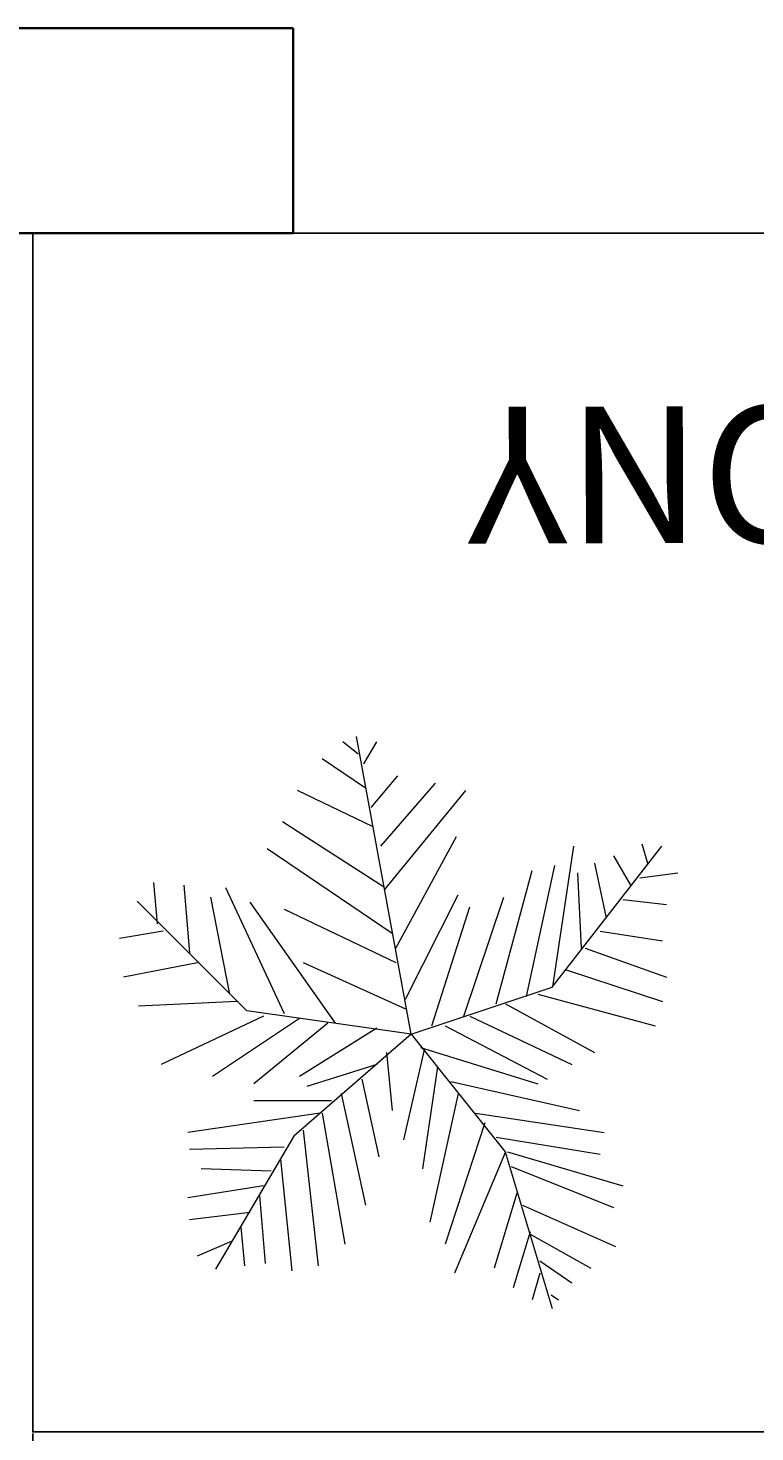
# Model space of a CAD drawing. Units: inches. Extents: x 4159 to 4826, y 299 to 1026.
# Tile 3 of 37: x 4268 to 4300, y 340 to 401. Entities that reach past the tile are written whole.
import ezdxf

# ---------------------------------------------------------------- set-up
doc = ezdxf.new("R2010")
doc.units = ezdxf.units.IN
for name, color, linetype, lineweight in [('A-ANNO-DIMS', 2, 'Continuous', 18), ('A-AREA-IDEN', 7, 'Continuous', 18), ('A-FLOR-BALC', 7, 'Continuous', 25), ('A-WALL', 7, 'Continuous', 35), ('L-PLNT', 94, 'Continuous', 13)]:
    doc.layers.add(name, color=color, linetype=linetype, lineweight=lineweight)
doc.styles.get("Standard").update_dxf_attribs({"font": 'arial.ttf'})
doc.dimstyles.get("Standard").update_dxf_attribs({"dimtxt": 0.18, "dimasz": 0.18, "dimexe": 0.18, "dimexo": 0.0625, "dimgap": 0.09, "dimtad": 0, "dimtih": 1, "dimtoh": 1, "dimdec": 4, "dimzin": 0, "dimdsep": 46, "dimtxsty": 'Standard', "dimcen": 0.09, "dimadec": 0, "dimazin": 0, "dimtfac": 1, "dimtdec": 4, "dimtofl": 0, "dimtmove": 0, "dimatfit": 3, "dimfxl": 1, "dimtolj": 1, "dimtzin": 0, "dimarcsym": 0})

# ---------------------------------------------------------------- blocks, each defined once
blk = doc.blocks.new('*U12')
for p, q in [((0, 0), (-10.5, 57)), ((-10.186, 53.64), (-13.084, 55.962)), ((-9.099, 51.782), (-6.563, 55.962)), ((-8.737, 47.138), (-17.069, 52.711)), ((-7.65, 43.423), (-2.578, 49.46)), ((-7.288, 39.707), (-21.778, 46.673)), ((-5.839, 35.992), (4.667, 48.067)), ((-5.114, 27.632), (10.463, 46.673)), ((-5.114, 28.097), (-24.676, 40.636)), ((-2.941, 16.486), (8.652, 37.85)), ((-3.665, 19.273), (-27.574, 35.527)), ((27, 9), (48, 36)), ((27.127, 9.056), (31.112, 35.992)), ((44.153, 36.456), (45.239, 32.741)), ((22.055, 7.198), (27.489, 32.277)), ((35.096, 32.741), (37.27, 22.524)), ((38.719, 34.134), (41.979, 28.561)), ((16.259, 5.805), (23.142, 31.348)), ((31.836, 30.883), (32.561, 16.486)), ((43.791, 29.954), (51.036, 30.883)), ((-48.585, 21.131), (-49.309, 29.026)), ((-43.513, 28.561), (-42.427, 15.558)), ((-35.544, 28.097), (-24.314, 3.947)), ((-31.5, 4.5), (-52.5, 25.5)), ((-38.442, 26.239), (-34.819, 7.663)), ((-14.533, 2.09), (-30.834, 25.31)), ((-1.129, 6.734), (9.014, 26.704)), ((3.942, 1.625), (11.187, 24.381)), ((10.101, 3.483), (17.708, 26.239)), ((40.53, 25.775), (48.862, 24.846)), ((-24.314, 23.917), (-2.941, 13.7)), ((-47.498, 19.737), (-55.83, 18.344)), ((36.183, 19.737), (48.137, 17.88)), ((33.285, 16.486), (48.862, 10.913)), ((-40.615, 13.7), (-55.105, 10.913)), ((-20.691, 13.7), (-1.129, 4.876)), ((29.662, 12.307), (48.137, 6.269)), ((0, 0), (27, 9)), ((-33.37, 6.269), (-52.207, 5.34)), ((18.07, 5.805), (35.096, -3.483)), ((24.229, 7.663), (46.688, 1.625)), ((-28.299, 3.483), (-47.86, -5.805)), ((-21.416, 3.018), (-38.079, -8.128)), ((0, 0), (-31.5, 4.5)), ((11.187, 3.483), (30.749, -5.805)), ((-15.982, 2.09), (-30.11, -9.521)), ((0, 0), (-22.5, -19.5)), ((-6.563, 1.161), (-21.416, -8.128)), ((0, 0), (18, -22.5)), ((6.478, 1.625), (26.04, -8.592)), ((1.769, -2.555), (24.229, -9.521)), ((-4.752, -3.483), (-3.665, -14.629)), ((2.493, -3.019), (-1.491, -20.202)), ((-6.563, -5.805), (-19.967, -9.985)), ((5.029, -6.27), (2.131, -25.775)), ((-9.461, -8.592), (-6.201, -23.453)), ((7.565, -9.056), (32.198, -14.629)), ((-15.257, -12.772), (-30.11, -12.772)), ((-13.446, -11.378), (-8.737, -32.741)), ((9.014, -11.378), (3.58, -35.992)), ((-17.431, -15.094), (-42.789, -18.809)), ((-17.069, -15.094), (-12.721, -40.172)), ((12.274, -15.094), (36.907, -18.809)), ((-20.691, -18.345), (-17.793, -44.352)), ((14.085, -16.951), (6.478, -40.172)), ((-22.5, -19.5), (-37.5, -45)), ((16.259, -19.738), (36.183, -22.989)), ((-24.314, -21.596), (-42.427, -22.06)), ((-25.038, -23.918), (-22.865, -45.281)), ((18.07, -22.524), (8.289, -45.745)), ((18, -22.5), (27, -52.5)), ((18.433, -22.524), (40.53, -29.026)), ((-26.849, -26.24), (-40.253, -25.775)), ((19.157, -25.311), (38.719, -33.206)), ((-28.299, -29.026), (-42.789, -31.348)), ((-29.023, -30.884), (-27.936, -43.887)), ((20.244, -30.419), (15.897, -44.816)), ((-30.834, -34.135), (-42.427, -35.528)), ((21.331, -32.741), (39.081, -40.636)), ((-32.646, -36.921), (-31.921, -44.352)), ((-34.457, -39.708), (-40.978, -42.494)), ((22.78, -37.85), (19.519, -48.532)), ((22.78, -38.314), (34.372, -44.816)), ((24.591, -43.423), (30.749, -47.603)), ((24.591, -45.745), (23.142, -50.854)), ((26.764, -49.925), (28.213, -50.854))]:
    blk.add_line(p, q)
blk = doc.blocks.new('*D44')
at = {"layer": 'A-ANNO-DIMS', "color": 0, "lineweight": -2, "transparency": 16777216}
for p, q in [((4287.263, 963.093), (4158.88, 963.093)), ((4159.06, 962.913), (4159.06, 647.826)), ((4159.06, 332.375), (4159.06, 647.462)), ((4447.248, 332.195), (4158.88, 332.195))]:
    blk.add_line(p, q, dxfattribs=at)
at = {"layer": 'A-ANNO-DIMS', "color": 0, "transparency": 16777216}
for points in [[(4159.03, 962.913), (4159.09, 962.913), (4159.06, 963.093)], [(4159.03, 332.375), (4159.09, 332.375), (4159.06, 332.195)]]:
    blk.add_solid(points, dxfattribs=at)
at = {"layer": 'Defpoints', "color": 0, "transparency": 16777216}
for p in [(4287.326, 963.093), (4159.06, 332.195), (4447.31, 332.195)]:
    blk.add_point(p, dxfattribs=at)
at = {"layer": 'A-ANNO-DIMS', "color": 0, "transparency": 16777216, "insert": (4159.06, 647.644), "char_height": 0.18, "attachment_point": 5}
blk.add_mtext('\\A1;630.9', dxfattribs=at)
blk = doc.blocks.new('*D46')
at = {"layer": 'A-ANNO-DIMS', "color": 0, "lineweight": -2, "transparency": 16777216}
for p, q in [((4192.31, 392.192), (4192.31, 298.765)), ((4447.31, 332.133), (4447.31, 298.765)), ((4192.49, 298.945), (4319.519, 298.945)), ((4447.13, 298.945), (4320.101, 298.945))]:
    blk.add_line(p, q, dxfattribs=at)
at = {"layer": 'A-ANNO-DIMS', "color": 0, "transparency": 16777216}
for points in [[(4192.49, 298.975), (4192.49, 298.915), (4192.31, 298.945)], [(4447.13, 298.975), (4447.13, 298.915), (4447.31, 298.945)]]:
    blk.add_solid(points, dxfattribs=at)
at = {"layer": 'Defpoints', "color": 0, "transparency": 16777216}
for p in [(4192.31, 392.254), (4447.31, 332.195), (4447.31, 298.945)]:
    blk.add_point(p, dxfattribs=at)
at = {"layer": 'A-ANNO-DIMS', "color": 0, "transparency": 16777216, "insert": (4319.81, 298.945), "char_height": 0.18, "attachment_point": 5}
blk.add_mtext('\\A1;255', dxfattribs=at)
blk = doc.blocks.new('*D52')
at = {"layer": 'A-ANNO-DIMS', "color": 0, "lineweight": -2, "transparency": 16777216}
for p, q in [((4192.31, 392.192), (4192.31, 298.765)), ((4267.89, 339.581), (4267.89, 298.765)), ((4192.49, 298.945), (4229.707, 298.945)), ((4267.71, 298.945), (4230.493, 298.945))]:
    blk.add_line(p, q, dxfattribs=at)
at = {"layer": 'A-ANNO-DIMS', "color": 0, "transparency": 16777216}
for points in [[(4192.49, 298.975), (4192.49, 298.915), (4192.31, 298.945)], [(4267.71, 298.975), (4267.71, 298.915), (4267.89, 298.945)]]:
    blk.add_solid(points, dxfattribs=at)
at = {"layer": 'Defpoints', "color": 0, "transparency": 16777216}
for p in [(4192.31, 392.254), (4267.89, 339.644), (4267.89, 298.945)]:
    blk.add_point(p, dxfattribs=at)
at = {"layer": 'A-ANNO-DIMS', "color": 0, "transparency": 16777216, "insert": (4230.1, 298.945), "char_height": 0.18, "attachment_point": 5}
blk.add_mtext('\\A1;75.58', dxfattribs=at)

msp = doc.modelspace()

# ---------------------------------------------------------------- linework, layer by layer
at = {"layer": 'A-FLOR-BALC'}
msp.add_lwpolyline([(4267.89, 392.254), (4383.821, 392.254), (4383.821, 339.644), (4267.89, 339.644)], close=True, dxfattribs=at)
at = {"layer": 'A-WALL'}
for p, q in [((4279.31, 401.254), (4201.31, 401.254)), ((4279.31, 401.254), (4279.31, 392.254)), ((4279.31, 392.254), (4192.31, 392.254))]:
    msp.add_line(p, q, dxfattribs=at)

# ---------------------------------------------------------------- block references
at = {"layer": 'L-PLNT', "xscale": 0.2292012274639507, "yscale": 0.2292012274639507, "zscale": 0.2292012274639507}
msp.add_blockref('*U12', (4284.496, 357.098), dxfattribs=at)

# ---------------------------------------------------------------- texts
at = {"layer": 'A-AREA-IDEN'}
msp.add_text("3' WIDE BALCONY", height=6, rotation=180.15208, dxfattribs=at).set_placement((4353.858, 384.806))

# ---------------------------------------------------------------- dimensions: what is measured, and where the dimension line sits
at = {"layer": 'A-ANNO-DIMS'}
dim = msp.add_linear_dim(base=(4159.06, 332.195), p1=(4287.326, 963.093), p2=(4447.31, 332.195), angle=90, dimstyle='Standard', override={"dimdec": 1, "dimlfac": 1, "dimrnd": 0, "dimzin": 0, "dimdsep": 46, "dimlunit": 2}, dxfattribs=at)
dim.commit()
dim.dimension.update_dxf_attribs({"geometry": '*D44', "text_midpoint": (4159.06, 647.644)})
for base, p2, override, picture, middle in [((4447.31, 298.945), (4447.31, 332.195), {"dimdec": 0, "dimlfac": 1, "dimrnd": 0, "dimzin": 0, "dimdsep": 46, "dimlunit": 2}, '*D46', (4319.81, 298.945)), ((4267.89, 298.945), (4267.89, 339.644), {"dimdec": 2, "dimlfac": 1, "dimrnd": 0, "dimzin": 0, "dimdsep": 46, "dimlunit": 2}, '*D52', (4230.1, 298.945))]:
    dim = msp.add_linear_dim(base=base, p1=(4192.31, 392.254), p2=p2, dimstyle='Standard', override=override, dxfattribs=at)
    dim.commit()
    dim.dimension.update_dxf_attribs({"geometry": picture, "text_midpoint": middle})

doc.saveas('drawing.dxf')
